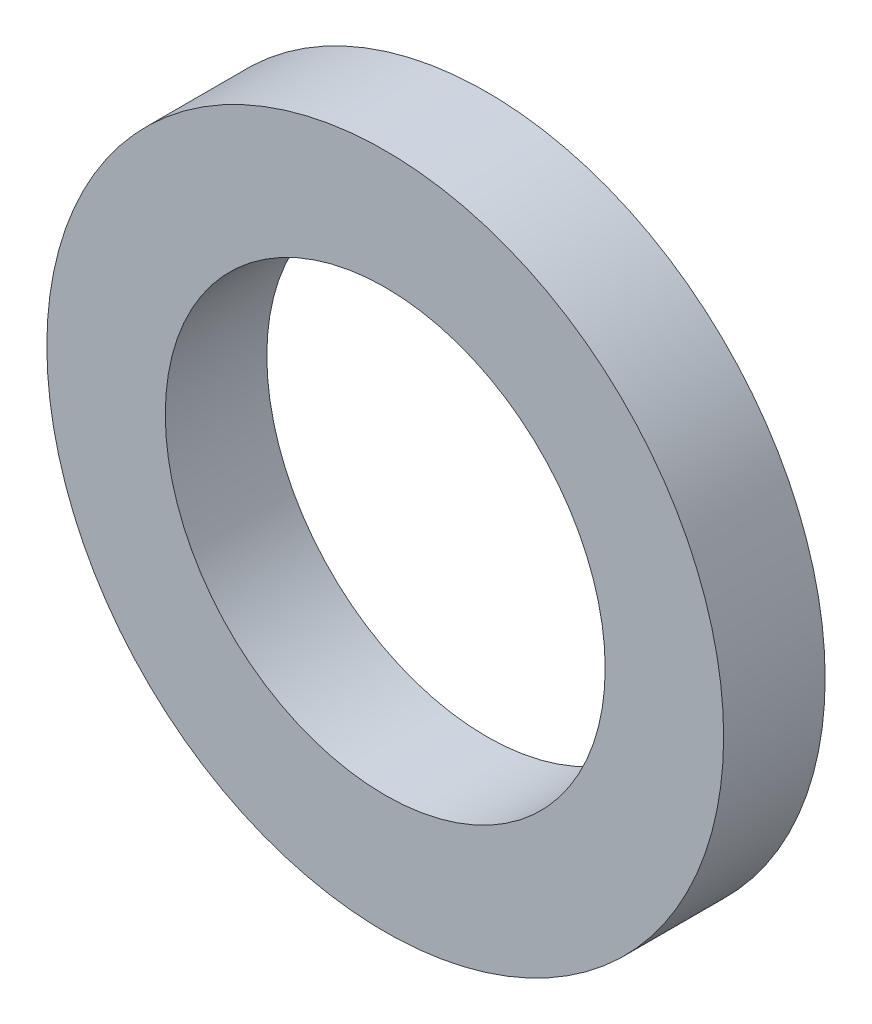
from build123d import *

# Parameters (mm, degrees)
WASHER_PROFILE_20X_13_R   = 10
WASHER_PROFILE_20X_13_R_2 = 6.5
WASHER_BODY_3MM_DEPTH     = 3


with BuildPart() as part:
    # Washer Profile Ø20xØ13 → Washer Body 3mm (new body)
    with BuildSketch(Plane.XY):
        Circle(WASHER_PROFILE_20X_13_R)
        Circle(WASHER_PROFILE_20X_13_R_2, mode=Mode.SUBTRACT)
    extrude(amount=WASHER_BODY_3MM_DEPTH)


solid = part.part
